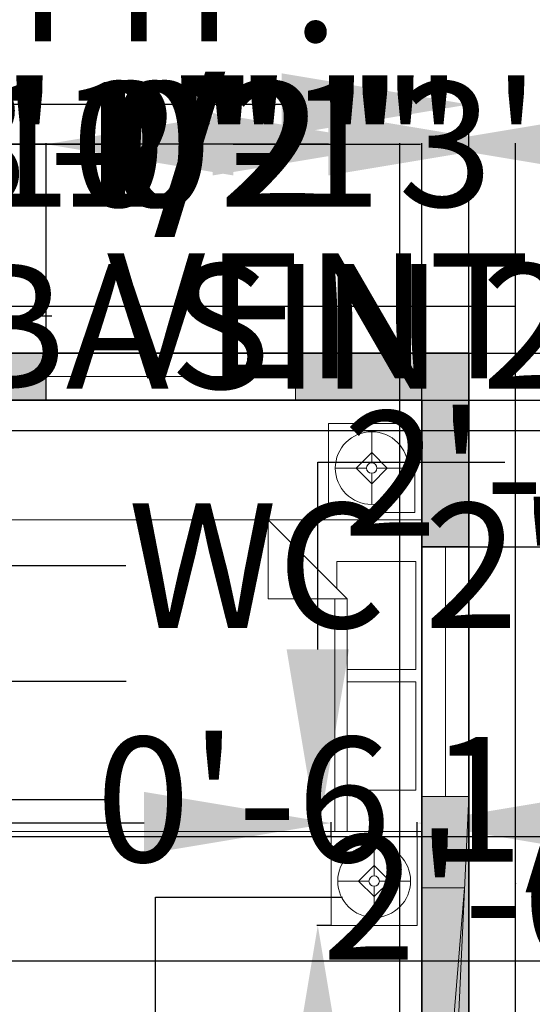
# Model space of a CAD drawing. Units: inches. Extents: x 2838 to 4029, y 1041 to 1915.
# Tile 13 of 16: x 3541 to 3640, y 1546 to 1735. Entities that reach past the tile are written whole.
import ezdxf

# ---------------------------------------------------------------- set-up
doc = ezdxf.new("R2010")
doc.units = ezdxf.units.IN
doc.header["$MEASUREMENT"] = 0
for name, color, linetype, lineweight in [('A-ANNO-DIMS', 2, 'Continuous', 18), ('A-FLOR', 7, 'Continuous', 25), ('A-FURN', 8, 'Continuous', 18), ('A-GLAZ', 4, 'Continuous', 18), ('A-REFR', 8, 'Continuous', 13), ('A-WALL', 7, 'Continuous', 35), ('A-WALL-PATT', 252, 'Continuous', 13)]:
    doc.layers.add(name, color=color, linetype=linetype, lineweight=lineweight)
doc.styles.get("Standard").update_dxf_attribs({"font": 'arial.ttf'})
doc.dimstyles.get("Standard").update_dxf_attribs({"dimtxt": 24, "dimasz": 36, "dimexe": 0.18, "dimexo": 0.0625, "dimgap": 0.09, "dimtad": 0, "dimtih": 1, "dimtoh": 1, "dimdec": 0, "dimzin": 0, "dimdsep": 46, "dimlunit": 3, "dimtxsty": 'Standard', "dimcen": 0.09, "dimadec": 0, "dimazin": 0, "dimtfac": 1, "dimtdec": 0, "dimtofl": 0, "dimtmove": 0, "dimatfit": 3, "dimfxl": 1, "dimtolj": 1, "dimtzin": 0, "dimarcsym": 0})

# ---------------------------------------------------------------- blocks, each defined once
blk = doc.blocks.new('Bed - Queen')
for p, q in [((0, -80.00003), (0, 0)), ((0, 0), (59.99999, 0)), ((59.99999, 0), (59.99999, -80.00003)), ((7.99999, -1.2), (28.79998, -1.2)), ((7.99999, -14.4), (7.99999, -1.2)), ((28.79998, -1.2), (28.79998, -14.4)), ((31.19999, -1.2), (51.99999, -1.2)), ((31.19999, -14.4), (31.19999, -1.2)), ((51.99999, -1.2), (51.99999, -16.4)), ((0, -14.4), (44.8, -14.4)), ((59.99999, -29.6), (44.8, -14.4)), ((44.8, -14.4), (44.8, -29.6)), ((44.8, -16.8), (0, -16.8)), ((51.99999, -16.4), (46.79936, -16.4)), ((44.8, -29.6), (59.99999, -29.6)), ((59.99999, -80.00003), (0, -80.00003))]:
    blk.add_line(p, q)
blk = doc.blocks.new('*D17')
at = {"layer": 'A-ANNO-DIMS', "color": 0, "lineweight": -2, "transparency": 16777216}
for p, q in [((3627.79, 1671.3), (3713.18, 1671.3)), ((3713, 1635.3), (3713, 1443.64)), ((3713, 1227.3), (3713, 1418.95)), ((3627.79, 1191.3), (3713.18, 1191.3))]:
    blk.add_line(p, q, dxfattribs=at)
at = {"layer": 'A-ANNO-DIMS', "color": 0, "transparency": 16777216}
for points in [[(3707, 1635.3), (3719, 1635.3), (3713, 1671.3)], [(3707, 1227.3), (3719, 1227.3), (3713, 1191.3)]]:
    blk.add_solid(points, dxfattribs=at)
at = {"layer": 'Defpoints', "color": 0, "transparency": 16777216}
for p in [(3627.73, 1671.3), (3627.73, 1191.3), (3713, 1191.3)]:
    blk.add_point(p, dxfattribs=at)
at = {"layer": 'A-ANNO-DIMS', "color": 0, "transparency": 16777216, "insert": (3713, 1431.3), "char_height": 24, "attachment_point": 5}
blk.add_mtext("\\A1;40'", dxfattribs=at)
blk = doc.blocks.new('*D18')
at = {"layer": 'A-ANNO-DIMS', "color": 0, "lineweight": -2, "transparency": 16777216}
for p, q in [((3267.73, 1671.36), (3267.73, 1719.35)), ((3303.73, 1719.17), (3427.28, 1719.17)), ((3591.73, 1719.17), (3468.18, 1719.17)), ((3627.73, 1671.36), (3627.73, 1719.35))]:
    blk.add_line(p, q, dxfattribs=at)
at = {"layer": 'A-ANNO-DIMS', "color": 0, "transparency": 16777216}
for points in [[(3303.73, 1725.17), (3303.73, 1713.17), (3267.73, 1719.17)], [(3591.73, 1725.17), (3591.73, 1713.17), (3627.73, 1719.17)]]:
    blk.add_solid(points, dxfattribs=at)
at = {"layer": 'Defpoints', "color": 0, "transparency": 16777216}
for p in [(3267.73, 1719.17), (3267.73, 1671.3), (3627.73, 1671.3)]:
    blk.add_point(p, dxfattribs=at)
at = {"layer": 'A-ANNO-DIMS', "color": 0, "transparency": 16777216, "insert": (3447.73, 1719.17), "char_height": 24, "attachment_point": 5}
blk.add_mtext("\\A1;30'", dxfattribs=at)
blk = doc.blocks.new('WIN-48')
blk.add_line((4.5, 48), (4.5, 0))
blk.add_lwpolyline([(0, 48), (9, 48), (9, 0), (0, 0)], close=True)
blk = doc.blocks.new('Lamp - Table')
for p, q in [((0, 7), (0, 1)), ((0, 3), (-3, 0)), ((3, 0), (0, 3)), ((-1, 0), (-7, 0)), ((-3, 0), (0, -3)), ((0, -3), (3, 0)), ((1, 0), (7, 0)), ((0, -1), (0, -7))]:
    blk.add_line(p, q)
for radius in [7, 1]:
    blk.add_circle((0, 0), radius)
blk = doc.blocks.new('NIGHTSTAND-WITH-LAMP')
blk.add_lwpolyline([(0, 17.15), (16.57, 17.15), (16.57, 0), (0, 0)], close=True)
blk.add_blockref('Lamp - Table', (8.28, 8.57))
blk = doc.blocks.new('*D27')
at = {"layer": 'A-ANNO-DIMS', "color": 0, "lineweight": -2, "transparency": 16777216}
for p, q in [((3598.68, 1614.31), (3598.68, 1650.31)), ((3598.68, 1650.31), (3634.68, 1650.31)), ((3601.19, 1578.31), (3598.5, 1578.31)), ((3601.19, 1561.16), (3598.5, 1561.16)), ((3598.68, 1525.16), (3598.68, 1489.16))]:
    blk.add_line(p, q, dxfattribs=at)
at = {"layer": 'A-ANNO-DIMS', "color": 0, "transparency": 16777216}
for points in [[(3592.68, 1614.31), (3604.68, 1614.31), (3598.68, 1578.31)], [(3592.68, 1525.16), (3604.68, 1525.16), (3598.68, 1561.16)]]:
    blk.add_solid(points, dxfattribs=at)
at = {"layer": 'Defpoints', "color": 0, "transparency": 16777216}
for p in [(3598.68, 1578.31), (3601.25, 1578.31), (3601.25, 1561.16)]:
    blk.add_point(p, dxfattribs=at)
at = {"layer": 'A-ANNO-DIMS', "color": 0, "transparency": 16777216, "insert": (3820.96, 1650.31), "char_height": 24, "attachment_point": 5}
blk.add_mtext('\\A1;NIGHTSTAND 1\'-5" TYP.', dxfattribs=at)
blk = doc.blocks.new('*D28')
at = {"layer": 'A-ANNO-DIMS', "color": 0, "lineweight": -2, "transparency": 16777216}
for p, q in [((3565.25, 1580.88), (3529.25, 1580.88)), ((3601.25, 1578.37), (3601.25, 1581.06)), ((3617.82, 1578.37), (3617.82, 1581.06)), ((3653.82, 1580.88), (3689.82, 1580.88))]:
    blk.add_line(p, q, dxfattribs=at)
at = {"layer": 'A-ANNO-DIMS', "color": 0, "transparency": 16777216}
for points in [[(3565.25, 1586.88), (3565.25, 1574.88), (3601.25, 1580.88)], [(3653.82, 1586.88), (3653.82, 1574.88), (3617.82, 1580.88)]]:
    blk.add_solid(points, dxfattribs=at)
at = {"layer": 'Defpoints', "color": 0, "transparency": 16777216}
for p in [(3617.82, 1580.88), (3601.25, 1578.31), (3617.82, 1578.31)]:
    blk.add_point(p, dxfattribs=at)
at = {"layer": 'A-ANNO-DIMS', "color": 0, "transparency": 16777216, "insert": (3789.89, 1580.88), "char_height": 24, "attachment_point": 5}
blk.add_mtext('\\A1;1\'-4 1/2" TYP.', dxfattribs=at)
blk = doc.blocks.new('*D36')
at = {"layer": 'A-ANNO-DIMS', "color": 0, "lineweight": -2, "transparency": 16777216}
for p, q in [((3481.95, 1586.87), (3481.95, 1585.25)), ((3488.45, 1586.87), (3488.45, 1585.25)), ((3445.95, 1585.43), (3409.95, 1585.43)), ((3524.45, 1585.43), (3560.45, 1585.43))]:
    blk.add_line(p, q, dxfattribs=at)
at = {"layer": 'A-ANNO-DIMS', "color": 0, "transparency": 16777216}
for points in [[(3445.95, 1591.43), (3445.95, 1579.43), (3481.95, 1585.43)], [(3524.45, 1591.43), (3524.45, 1579.43), (3488.45, 1585.43)]]:
    blk.add_solid(points, dxfattribs=at)
at = {"layer": 'Defpoints', "color": 0, "transparency": 16777216}
for p in [(3481.95, 1586.93), (3488.45, 1586.93), (3488.45, 1585.43)]:
    blk.add_point(p, dxfattribs=at)
at = {"layer": 'A-ANNO-DIMS', "color": 0, "transparency": 16777216, "insert": (3620.4, 1585.43), "char_height": 24, "attachment_point": 5}
blk.add_mtext('\\A1;0\'-6 1/2"', dxfattribs=at)
blk = doc.blocks.new('*D39')
at = {"layer": 'A-ANNO-DIMS', "color": 0, "lineweight": -2, "transparency": 16777216}
for p, q in [((3391.52, 1678.5), (3355.52, 1678.5)), ((3427.52, 1671.36), (3427.52, 1678.68)), ((3475.52, 1671.36), (3475.52, 1678.68)), ((3511.52, 1678.5), (3547.52, 1678.5))]:
    blk.add_line(p, q, dxfattribs=at)
at = {"layer": 'A-ANNO-DIMS', "color": 0, "transparency": 16777216}
for points in [[(3391.52, 1684.5), (3391.52, 1672.5), (3427.52, 1678.5)], [(3511.52, 1684.5), (3511.52, 1672.5), (3475.52, 1678.5)]]:
    blk.add_solid(points, dxfattribs=at)
at = {"layer": 'Defpoints', "color": 0, "transparency": 16777216}
for p in [(3475.52, 1678.5), (3427.52, 1671.3), (3475.52, 1671.3)]:
    blk.add_point(p, dxfattribs=at)
at = {"layer": 'A-ANNO-DIMS', "color": 0, "transparency": 16777216, "insert": (3732.24, 1678.5), "char_height": 24, "attachment_point": 5}
blk.add_mtext('\\A1;VENT BLOCK 4\'-0" TYP.', dxfattribs=at)
blk = doc.blocks.new('*D40')
at = {"layer": 'A-ANNO-DIMS', "color": 0, "lineweight": -2, "transparency": 16777216}
for p, q in [((3420.32, 1707.3), (3420.32, 1743.3)), ((3420.32, 1743.3), (3456.32, 1743.3)), ((3427.46, 1671.3), (3420.14, 1671.3)), ((3427.46, 1662.3), (3420.14, 1662.3)), ((3420.32, 1626.3), (3420.32, 1590.3))]:
    blk.add_line(p, q, dxfattribs=at)
at = {"layer": 'A-ANNO-DIMS', "color": 0, "transparency": 16777216}
for points in [[(3414.32, 1707.3), (3426.32, 1707.3), (3420.32, 1671.3)], [(3414.32, 1626.3), (3426.32, 1626.3), (3420.32, 1662.3)]]:
    blk.add_solid(points, dxfattribs=at)
at = {"layer": 'Defpoints', "color": 0, "transparency": 16777216}
for p in [(3420.32, 1671.3), (3427.52, 1671.3), (3427.52, 1662.3)]:
    blk.add_point(p, dxfattribs=at)
at = {"layer": 'A-ANNO-DIMS', "color": 0, "transparency": 16777216, "insert": (3529.56, 1743.3), "char_height": 24, "attachment_point": 5}
blk.add_mtext('\\A1;0\'-9" TYP.', dxfattribs=at)
blk = doc.blocks.new('*D41')
at = {"layer": 'A-ANNO-DIMS', "color": 0, "lineweight": -2, "transparency": 16777216}
for p, q in [((3284.24, 1506.2), (3284.24, 1496.56)), ((3347.73, 1506.2), (3347.73, 1496.56)), ((3248.24, 1496.74), (3212.24, 1496.74)), ((3383.73, 1496.74), (3419.73, 1496.74))]:
    blk.add_line(p, q, dxfattribs=at)
at = {"layer": 'A-ANNO-DIMS', "color": 0, "transparency": 16777216}
for points in [[(3248.24, 1502.74), (3248.24, 1490.74), (3284.24, 1496.74)], [(3383.73, 1502.74), (3383.73, 1490.74), (3347.73, 1496.74)]]:
    blk.add_solid(points, dxfattribs=at)
at = {"layer": 'Defpoints', "color": 0, "transparency": 16777216}
for p in [(3284.24, 1506.26), (3347.73, 1506.26), (3347.73, 1496.74)]:
    blk.add_point(p, dxfattribs=at)
at = {"layer": 'A-ANNO-DIMS', "color": 0, "transparency": 16777216, "insert": (3624.81, 1496.74), "char_height": 24, "attachment_point": 5}
blk.add_mtext('\\A1;WARDROBE 5\'-3 1/2" TYP.', dxfattribs=at)
blk = doc.blocks.new('*D45')
at = {"layer": 'A-ANNO-DIMS', "color": 0, "lineweight": -2, "transparency": 16777216}
for p, q in [((3456.69, 1635.35), (3456.69, 1630.27)), ((3489.73, 1635.35), (3489.73, 1630.27)), ((3420.69, 1630.45), (3384.69, 1630.45)), ((3525.73, 1630.45), (3561.73, 1630.45))]:
    blk.add_line(p, q, dxfattribs=at)
at = {"layer": 'A-ANNO-DIMS', "color": 0, "transparency": 16777216}
for points in [[(3420.69, 1636.45), (3420.69, 1624.45), (3456.69, 1630.45)], [(3525.73, 1636.45), (3525.73, 1624.45), (3489.73, 1630.45)]]:
    blk.add_solid(points, dxfattribs=at)
at = {"layer": 'Defpoints', "color": 0, "transparency": 16777216}
for p in [(3456.69, 1635.41), (3489.73, 1635.41), (3489.73, 1630.45)]:
    blk.add_point(p, dxfattribs=at)
at = {"layer": 'A-ANNO-DIMS', "color": 0, "transparency": 16777216, "insert": (3626.8, 1630.45), "char_height": 24, "attachment_point": 5}
blk.add_mtext('\\A1;WC 2\'-9"', dxfattribs=at)
blk = doc.blocks.new('*D47')
at = {"layer": 'A-ANNO-DIMS', "color": 0, "lineweight": -2, "transparency": 16777216}
for p, q in [((3493.47, 1640.5), (3493.47, 1676.5)), ((3493.47, 1676.5), (3529.47, 1676.5)), ((3489.85, 1604.5), (3493.65, 1604.5)), ((3489.85, 1579.95), (3493.65, 1579.95)), ((3493.47, 1543.95), (3493.47, 1507.95))]:
    blk.add_line(p, q, dxfattribs=at)
at = {"layer": 'A-ANNO-DIMS', "color": 0, "transparency": 16777216}
for points in [[(3487.47, 1640.5), (3499.47, 1640.5), (3493.47, 1604.5)], [(3487.47, 1543.95), (3499.47, 1543.95), (3493.47, 1579.95)]]:
    blk.add_solid(points, dxfattribs=at)
at = {"layer": 'Defpoints', "color": 0, "transparency": 16777216}
for p in [(3489.78, 1604.5), (3493.47, 1604.5), (3489.78, 1579.95)]:
    blk.add_point(p, dxfattribs=at)
at = {"layer": 'A-ANNO-DIMS', "color": 0, "transparency": 16777216, "insert": (3643.85, 1676.5), "char_height": 24, "attachment_point": 5}
blk.add_mtext('\\A1;BASIN 2\'-0 1/2"', dxfattribs=at)
blk = doc.blocks.new('*D48')
at = {"layer": 'A-ANNO-DIMS', "color": 0, "lineweight": -2, "transparency": 16777216}
for p, q in [((3433.65, 1608.18), (3397.65, 1608.18)), ((3469.65, 1604.56), (3469.65, 1608.36)), ((3489.78, 1604.56), (3489.78, 1608.36)), ((3525.78, 1608.18), (3561.78, 1608.18))]:
    blk.add_line(p, q, dxfattribs=at)
at = {"layer": 'A-ANNO-DIMS', "color": 0, "transparency": 16777216}
for points in [[(3433.65, 1614.18), (3433.65, 1602.18), (3469.65, 1608.18)], [(3525.78, 1614.18), (3525.78, 1602.18), (3489.78, 1608.18)]]:
    blk.add_solid(points, dxfattribs=at)
at = {"layer": 'Defpoints', "color": 0, "transparency": 16777216}
for p in [(3469.65, 1608.18), (3469.65, 1604.5), (3489.78, 1604.5)]:
    blk.add_point(p, dxfattribs=at)
at = {"layer": 'A-ANNO-DIMS', "color": 0, "transparency": 16777216, "insert": (3366.79, 1608.18), "char_height": 24, "attachment_point": 5}
blk.add_mtext('\\A1;1\'-8"', dxfattribs=at)
blk = doc.blocks.new('*D55')
at = {"layer": 'A-ANNO-DIMS', "color": 0, "lineweight": -2, "transparency": 16777216}
for p, q in [((3491.76, 1499.78), (3455.76, 1499.78)), ((3527.76, 1494.67), (3527.76, 1499.96)), ((3562.26, 1494.67), (3562.26, 1499.96)), ((3598.26, 1499.78), (3634.26, 1499.78))]:
    blk.add_line(p, q, dxfattribs=at)
at = {"layer": 'A-ANNO-DIMS', "color": 0, "transparency": 16777216}
for points in [[(3491.76, 1505.78), (3491.76, 1493.78), (3527.76, 1499.78)], [(3598.26, 1505.78), (3598.26, 1493.78), (3562.26, 1499.78)]]:
    blk.add_solid(points, dxfattribs=at)
at = {"layer": 'Defpoints', "color": 0, "transparency": 16777216}
for p in [(3527.76, 1499.78), (3527.76, 1494.6), (3562.26, 1494.6)]:
    blk.add_point(p, dxfattribs=at)
at = {"layer": 'A-ANNO-DIMS', "color": 0, "transparency": 16777216, "insert": (3260.33, 1499.78), "char_height": 24, "attachment_point": 5}
blk.add_mtext('\\A1;BASE CABINET 2\'-10 1/2"', dxfattribs=at)
blk = doc.blocks.new('*D56')
at = {"layer": 'A-ANNO-DIMS', "color": 0, "lineweight": -2, "transparency": 16777216}
for p, q in [((3567.44, 1530.6), (3567.44, 1566.6)), ((3567.44, 1566.6), (3603.44, 1566.6)), ((3562.33, 1494.6), (3567.62, 1494.6)), ((3562.33, 1470.6), (3567.62, 1470.6)), ((3567.44, 1434.6), (3567.44, 1398.6))]:
    blk.add_line(p, q, dxfattribs=at)
at = {"layer": 'A-ANNO-DIMS', "color": 0, "transparency": 16777216}
for points in [[(3561.44, 1530.6), (3573.44, 1530.6), (3567.44, 1494.6)], [(3561.44, 1434.6), (3573.44, 1434.6), (3567.44, 1470.6)]]:
    blk.add_solid(points, dxfattribs=at)
at = {"layer": 'Defpoints', "color": 0, "transparency": 16777216}
for p in [(3562.26, 1494.6), (3567.44, 1494.6), (3562.26, 1470.6)]:
    blk.add_point(p, dxfattribs=at)
at = {"layer": 'A-ANNO-DIMS', "color": 0, "transparency": 16777216, "insert": (3635.63, 1566.6), "char_height": 24, "attachment_point": 5}
blk.add_mtext('\\A1;2\'-0"', dxfattribs=at)
blk = doc.blocks.new('*D68')
at = {"layer": 'A-ANNO-DIMS', "color": 0, "lineweight": -2, "transparency": 16777216}
for p, q in [((3258.73, 1680.36), (3258.73, 1711.7)), ((3294.73, 1711.52), (3406.43, 1711.52)), ((3600.73, 1711.52), (3489.04, 1711.52)), ((3636.73, 1680.36), (3636.73, 1711.7))]:
    blk.add_line(p, q, dxfattribs=at)
at = {"layer": 'A-ANNO-DIMS', "color": 0, "transparency": 16777216}
for points in [[(3294.73, 1717.52), (3294.73, 1705.52), (3258.73, 1711.52)], [(3600.73, 1717.52), (3600.73, 1705.52), (3636.73, 1711.52)]]:
    blk.add_solid(points, dxfattribs=at)
at = {"layer": 'Defpoints', "color": 0, "transparency": 16777216}
for p in [(3636.73, 1711.52), (3258.73, 1680.3), (3636.73, 1680.3)]:
    blk.add_point(p, dxfattribs=at)
at = {"layer": 'A-ANNO-DIMS', "color": 0, "transparency": 16777216, "insert": (3447.73, 1711.52), "char_height": 24, "attachment_point": 5}
blk.add_mtext('\\A1;31\'-6"', dxfattribs=at)
blk = doc.blocks.new('*D73')
at = {"layer": 'A-ANNO-DIMS', "color": 0, "lineweight": -2, "transparency": 16777216}
for p, q in [((3425.038746, 1711.522346), (3389.038746, 1711.522346)), ((3461.038746, 1200.359846), (3461.038746, 1711.702346)), ((3618.731626, 1200.359846), (3618.731626, 1711.702346)), ((3654.731626, 1711.522346), (3690.731626, 1711.522346))]:
    blk.add_line(p, q, dxfattribs=at)
at = {"layer": 'A-ANNO-DIMS', "color": 0, "transparency": 16777216}
for points in [[(3425.038746, 1717.522346), (3425.038746, 1705.522346), (3461.038746, 1711.522346)], [(3654.731626, 1717.522346), (3654.731626, 1705.522346), (3618.731626, 1711.522346)]]:
    blk.add_solid(points, dxfattribs=at)
at = {"layer": 'Defpoints', "color": 0, "transparency": 16777216}
for p in [(3618.731626, 1711.522346), (3461.038746, 1200.297346), (3618.731626, 1200.297346)]:
    blk.add_point(p, dxfattribs=at)
at = {"layer": 'A-ANNO-DIMS', "color": 0, "transparency": 16777216, "insert": (3539.885186, 1711.522346), "char_height": 24, "attachment_point": 5}
blk.add_mtext('\\A1;13\'-1 1/2"', dxfattribs=at)
blk = doc.blocks.new('*D78')
at = {"layer": 'A-ANNO-DIMS', "color": 0, "lineweight": -2, "transparency": 16777216}
for p, q in [((3667.956626, 1590.394218), (3667.956626, 1626.394218)), ((3498.794126, 1554.394218), (3668.136626, 1554.394218)), ((3498.638013, 1506.394218), (3668.136626, 1506.394218)), ((3667.956626, 1470.394218), (3667.956626, 1434.394218))]:
    blk.add_line(p, q, dxfattribs=at)
at = {"layer": 'A-ANNO-DIMS', "color": 0, "transparency": 16777216}
for points in [[(3661.956626, 1590.394218), (3673.956626, 1590.394218), (3667.956626, 1554.394218)], [(3661.956626, 1470.394218), (3673.956626, 1470.394218), (3667.956626, 1506.394218)]]:
    blk.add_solid(points, dxfattribs=at)
at = {"layer": 'Defpoints', "color": 0, "transparency": 16777216}
for p in [(3498.731626, 1554.394218), (3667.956626, 1554.394218), (3498.575513, 1506.394218)]:
    blk.add_point(p, dxfattribs=at)
at = {"layer": 'A-ANNO-DIMS', "color": 0, "transparency": 16777216, "insert": (3667.956626, 1530.394218), "char_height": 24, "attachment_point": 5}
blk.add_mtext('\\A1;4\'-0"', dxfattribs=at)
blk = doc.blocks.new('*D79')
at = {"layer": 'A-ANNO-DIMS', "color": 0, "lineweight": -2, "transparency": 16777216}
for p, q in [((3379.05, 1400.64), (3379.05, 1711.7)), ((3415.05, 1711.52), (3418.63, 1711.52)), ((3454.63, 1398.31), (3454.63, 1711.7)), ((3454.63, 1711.52), (3490.63, 1711.52))]:
    blk.add_line(p, q, dxfattribs=at)
at = {"layer": 'A-ANNO-DIMS', "color": 0, "transparency": 16777216}
for points in [[(3415.05, 1717.52), (3415.05, 1705.52), (3379.05, 1711.52)], [(3418.63, 1717.52), (3418.63, 1705.52), (3454.63, 1711.52)]]:
    blk.add_solid(points, dxfattribs=at)
at = {"layer": 'Defpoints', "color": 0, "transparency": 16777216}
for p in [(3454.63, 1711.52), (3379.05, 1400.57), (3454.63, 1398.25)]:
    blk.add_point(p, dxfattribs=at)
at = {"layer": 'A-ANNO-DIMS', "color": 0, "transparency": 16777216, "insert": (3550.65, 1711.52), "char_height": 24, "attachment_point": 5}
blk.add_mtext('\\A1;6\'-3 1/2"', dxfattribs=at)
blk = doc.blocks.new('*D82')
at = {"layer": 'A-ANNO-DIMS', "color": 0, "lineweight": -2, "transparency": 16777216}
for p, q in [((3405.73, 1573.06), (3405.73, 1081.89)), ((3441.73, 1569.23), (3441.73, 1081.89)), ((3369.73, 1082.07), (3333.73, 1082.07)), ((3477.73, 1082.07), (3513.73, 1082.07))]:
    blk.add_line(p, q, dxfattribs=at)
at = {"layer": 'A-ANNO-DIMS', "color": 0, "transparency": 16777216}
for points in [[(3369.73, 1088.07), (3369.73, 1076.07), (3405.73, 1082.07)], [(3477.73, 1088.07), (3477.73, 1076.07), (3441.73, 1082.07)]]:
    blk.add_solid(points, dxfattribs=at)
at = {"layer": 'Defpoints', "color": 0, "transparency": 16777216}
for p in [(3405.73, 1573.12), (3441.73, 1569.3), (3441.73, 1082.07)]:
    blk.add_point(p, dxfattribs=at)
at = {"layer": 'A-ANNO-DIMS', "color": 0, "transparency": 16777216, "insert": (3545.71, 1082.07), "char_height": 24, "attachment_point": 5}
blk.add_mtext('\\A1;3\'-0"', dxfattribs=at)
blk = doc.blocks.new('*D83')
at = {"layer": 'A-ANNO-DIMS', "color": 0, "lineweight": -2, "transparency": 16777216}
for p, q in [((3405.73, 1662.36), (3405.73, 1711.7)), ((3441.73, 1711.52), (3453.73, 1711.52)), ((3489.73, 1662.36), (3489.73, 1711.7)), ((3489.73, 1711.52), (3525.73, 1711.52))]:
    blk.add_line(p, q, dxfattribs=at)
at = {"layer": 'A-ANNO-DIMS', "color": 0, "transparency": 16777216}
for points in [[(3441.73, 1717.52), (3441.73, 1705.52), (3405.73, 1711.52)], [(3453.73, 1717.52), (3453.73, 1705.52), (3489.73, 1711.52)]]:
    blk.add_solid(points, dxfattribs=at)
at = {"layer": 'Defpoints', "color": 0, "transparency": 16777216}
for p in [(3489.73, 1711.52), (3405.73, 1662.3), (3489.73, 1662.3)]:
    blk.add_point(p, dxfattribs=at)
at = {"layer": 'A-ANNO-DIMS', "color": 0, "transparency": 16777216, "insert": (3557.62, 1711.52), "char_height": 24, "attachment_point": 5}
blk.add_mtext('\\A1;7\'-0"', dxfattribs=at)
blk = doc.blocks.new('*D84')
at = {"layer": 'A-ANNO-DIMS', "color": 0, "lineweight": -2, "transparency": 16777216}
for p, q in [((3667.96, 1662.3), (3667.96, 1698.3)), ((3667.96, 1698.3), (3703.96, 1698.3)), ((3489.79, 1662.3), (3668.14, 1662.3)), ((3667.96, 1614.3), (3667.96, 1626.3)), ((3489.79, 1578.3), (3668.14, 1578.3))]:
    blk.add_line(p, q, dxfattribs=at)
at = {"layer": 'A-ANNO-DIMS', "color": 0, "transparency": 16777216}
for points in [[(3661.96, 1626.3), (3673.96, 1626.3), (3667.96, 1662.3)], [(3661.96, 1614.3), (3673.96, 1614.3), (3667.96, 1578.3)]]:
    blk.add_solid(points, dxfattribs=at)
at = {"layer": 'Defpoints', "color": 0, "transparency": 16777216}
for p in [(3489.73, 1662.3), (3667.96, 1662.3), (3489.73, 1578.3)]:
    blk.add_point(p, dxfattribs=at)
at = {"layer": 'A-ANNO-DIMS', "color": 0, "transparency": 16777216, "insert": (3735.85, 1698.3), "char_height": 24, "attachment_point": 5}
blk.add_mtext('\\A1;7\'-0"', dxfattribs=at)
blk = doc.blocks.new('*D85')
at = {"layer": 'A-ANNO-DIMS', "color": 0, "lineweight": -2, "transparency": 16777216}
for p, q in [((3369.73, 1711.52), (3333.73, 1711.52)), ((3405.73, 1662.36), (3405.73, 1711.7)), ((3427.52, 1662.36), (3427.52, 1711.7)), ((3463.52, 1711.52), (3499.52, 1711.52))]:
    blk.add_line(p, q, dxfattribs=at)
at = {"layer": 'A-ANNO-DIMS', "color": 0, "transparency": 16777216}
for points in [[(3369.73, 1717.52), (3369.73, 1705.52), (3405.73, 1711.52)], [(3463.52, 1717.52), (3463.52, 1705.52), (3427.52, 1711.52)]]:
    blk.add_solid(points, dxfattribs=at)
at = {"layer": 'Defpoints', "color": 0, "transparency": 16777216}
for p in [(3427.52, 1711.52), (3405.73, 1662.3), (3427.52, 1662.3)]:
    blk.add_point(p, dxfattribs=at)
at = {"layer": 'A-ANNO-DIMS', "color": 0, "transparency": 16777216, "insert": (3539.7, 1711.52), "char_height": 24, "attachment_point": 5}
blk.add_mtext('\\A1;1\'-10"', dxfattribs=at)
blk = doc.blocks.new('*D86')
at = {"layer": 'A-ANNO-DIMS', "color": 0, "lineweight": -2, "transparency": 16777216}
for p, q in [((3391.52, 1711.52), (3355.52, 1711.52)), ((3427.52, 1671.36), (3427.52, 1711.7)), ((3451.52, 1671.36), (3451.52, 1711.7)), ((3487.52, 1711.52), (3523.52, 1711.52))]:
    blk.add_line(p, q, dxfattribs=at)
at = {"layer": 'A-ANNO-DIMS', "color": 0, "transparency": 16777216}
for points in [[(3391.52, 1717.52), (3391.52, 1705.52), (3427.52, 1711.52)], [(3487.52, 1717.52), (3487.52, 1705.52), (3451.52, 1711.52)]]:
    blk.add_solid(points, dxfattribs=at)
at = {"layer": 'Defpoints', "color": 0, "transparency": 16777216}
for p in [(3451.52, 1711.52), (3427.52, 1671.3), (3451.52, 1671.3)]:
    blk.add_point(p, dxfattribs=at)
at = {"layer": 'A-ANNO-DIMS', "color": 0, "transparency": 16777216, "insert": (3555.72, 1711.52), "char_height": 24, "attachment_point": 5}
blk.add_mtext('\\A1;2\'-0"', dxfattribs=at)
blk = doc.blocks.new('*D94')
at = {"layer": 'A-ANNO-DIMS', "color": 0, "lineweight": -2, "transparency": 16777216}
for p, q in [((3667.96, 1533.39), (3667.96, 1569.39)), ((3585.44, 1497.39), (3668.14, 1497.39)), ((3585.44, 1469.25), (3668.14, 1469.25)), ((3667.96, 1433.25), (3667.96, 1397.25))]:
    blk.add_line(p, q, dxfattribs=at)
at = {"layer": 'A-ANNO-DIMS', "color": 0, "transparency": 16777216}
for points in [[(3661.96, 1533.39), (3673.96, 1533.39), (3667.96, 1497.39)], [(3661.96, 1433.25), (3673.96, 1433.25), (3667.96, 1469.25)]]:
    blk.add_solid(points, dxfattribs=at)
at = {"layer": 'Defpoints', "color": 0, "transparency": 16777216}
for p in [(3585.37, 1497.39), (3585.37, 1469.25), (3667.96, 1469.25)]:
    blk.add_point(p, dxfattribs=at)
at = {"layer": 'A-ANNO-DIMS', "color": 0, "transparency": 16777216, "insert": (3667.96, 1483.32), "char_height": 24, "attachment_point": 5}
blk.add_mtext('\\A1;2\'-4"', dxfattribs=at)
blk = doc.blocks.new('*D96')
at = {"layer": 'A-ANNO-DIMS', "color": 0, "lineweight": -2, "transparency": 16777216}
for p, q in [((3462.73, 1711.52), (3426.73, 1711.52)), ((3498.73, 1662.36), (3498.73, 1711.7)), ((3546.42, 1662.36), (3546.42, 1711.7)), ((3582.42, 1711.52), (3618.42, 1711.52))]:
    blk.add_line(p, q, dxfattribs=at)
at = {"layer": 'A-ANNO-DIMS', "color": 0, "transparency": 16777216}
for points in [[(3462.73, 1717.52), (3462.73, 1705.52), (3498.73, 1711.52)], [(3582.42, 1717.52), (3582.42, 1705.52), (3546.42, 1711.52)]]:
    blk.add_solid(points, dxfattribs=at)
at = {"layer": 'Defpoints', "color": 0, "transparency": 16777216}
for p in [(3546.42, 1711.52), (3498.73, 1662.3), (3546.42, 1662.3)]:
    blk.add_point(p, dxfattribs=at)
at = {"layer": 'A-ANNO-DIMS', "color": 0, "transparency": 16777216, "insert": (3687.68, 1711.52), "char_height": 24, "attachment_point": 5}
blk.add_mtext('\\A1;3\'-11 1/2"', dxfattribs=at)
blk = doc.blocks.new('*D97')
at = {"layer": 'A-ANNO-DIMS', "color": 0, "lineweight": -2, "transparency": 16777216}
for p, q in [((3667.956626, 1698.297346), (3667.956626, 1734.297346)), ((3618.794126, 1662.297346), (3668.136626, 1662.297346)), ((3618.794126, 1634.032994), (3668.136626, 1634.032994)), ((3667.956626, 1598.032994), (3667.956626, 1562.032994))]:
    blk.add_line(p, q, dxfattribs=at)
at = {"layer": 'A-ANNO-DIMS', "color": 0, "transparency": 16777216}
for points in [[(3661.956626, 1698.297346), (3673.956626, 1698.297346), (3667.956626, 1662.297346)], [(3661.956626, 1598.032994), (3673.956626, 1598.032994), (3667.956626, 1634.032994)]]:
    blk.add_solid(points, dxfattribs=at)
at = {"layer": 'Defpoints', "color": 0, "transparency": 16777216}
for p in [(3618.731626, 1662.297346), (3618.731626, 1634.032994), (3667.956626, 1634.032994)]:
    blk.add_point(p, dxfattribs=at)
at = {"layer": 'A-ANNO-DIMS', "color": 0, "transparency": 16777216, "insert": (3667.956626, 1648.16517), "char_height": 24, "attachment_point": 5}
blk.add_mtext('\\A1;2\'-4 1/2"', dxfattribs=at)
blk = doc.blocks.new('*D101')
at = {"layer": 'A-ANNO-DIMS', "color": 0, "lineweight": -2, "transparency": 16777216}
for p, q in [((3425.04, 1711.52), (3389.04, 1711.52)), ((3461.04, 1200.36), (3461.04, 1711.7)), ((3486.18, 1200.36), (3486.18, 1711.7)), ((3522.18, 1711.52), (3558.18, 1711.52))]:
    blk.add_line(p, q, dxfattribs=at)
at = {"layer": 'A-ANNO-DIMS', "color": 0, "transparency": 16777216}
for points in [[(3425.04, 1717.52), (3425.04, 1705.52), (3461.04, 1711.52)], [(3522.18, 1717.52), (3522.18, 1705.52), (3486.18, 1711.52)]]:
    blk.add_solid(points, dxfattribs=at)
at = {"layer": 'Defpoints', "color": 0, "transparency": 16777216}
for p in [(3486.18, 1711.52), (3461.04, 1200.3), (3486.18, 1200.3)]:
    blk.add_point(p, dxfattribs=at)
at = {"layer": 'A-ANNO-DIMS', "color": 0, "transparency": 16777216, "insert": (3590.37, 1711.52), "char_height": 24, "attachment_point": 5}
blk.add_mtext('\\A1;2\'-1"', dxfattribs=at)
blk = doc.blocks.new('*D102')
at = {"layer": 'A-ANNO-DIMS', "color": 0, "lineweight": -2, "transparency": 16777216}
for p, q in [((3667.96, 1698.3), (3667.96, 1734.3)), ((3667.96, 1734.3), (3703.96, 1734.3)), ((3489.79, 1662.3), (3668.14, 1662.3)), ((3489.79, 1656.41), (3668.14, 1656.41)), ((3667.96, 1620.41), (3667.96, 1584.41))]:
    blk.add_line(p, q, dxfattribs=at)
at = {"layer": 'A-ANNO-DIMS', "color": 0, "transparency": 16777216}
for points in [[(3661.96, 1698.3), (3673.96, 1698.3), (3667.96, 1662.3)], [(3661.96, 1620.41), (3673.96, 1620.41), (3667.96, 1656.41)]]:
    blk.add_solid(points, dxfattribs=at)
at = {"layer": 'Defpoints', "color": 0, "transparency": 16777216}
for p in [(3489.73, 1662.3), (3667.96, 1662.3), (3489.73, 1656.41)]:
    blk.add_point(p, dxfattribs=at)
at = {"layer": 'A-ANNO-DIMS', "color": 0, "transparency": 16777216, "insert": (3735.95, 1734.3), "char_height": 24, "attachment_point": 5}
blk.add_mtext('\\A1;0\'-6"', dxfattribs=at)
blk = doc.blocks.new('*D104')
at = {"layer": 'A-ANNO-DIMS', "color": 0, "lineweight": -2, "transparency": 16777216}
for p, q in [((3667.956626, 1533.394218), (3667.956626, 1569.394218)), ((3618.794126, 1497.394218), (3668.136626, 1497.394218)), ((3614.522024, 1472.357294), (3668.136626, 1472.357294)), ((3667.956626, 1436.357294), (3667.956626, 1400.357294))]:
    blk.add_line(p, q, dxfattribs=at)
at = {"layer": 'A-ANNO-DIMS', "color": 0, "transparency": 16777216}
for points in [[(3661.956626, 1533.394218), (3673.956626, 1533.394218), (3667.956626, 1497.394218)], [(3661.956626, 1436.357294), (3673.956626, 1436.357294), (3667.956626, 1472.357294)]]:
    blk.add_solid(points, dxfattribs=at)
at = {"layer": 'Defpoints', "color": 0, "transparency": 16777216}
for p in [(3618.731626, 1497.394218), (3614.459524, 1472.357294), (3667.956626, 1472.357294)]:
    blk.add_point(p, dxfattribs=at)
at = {"layer": 'A-ANNO-DIMS', "color": 0, "transparency": 16777216, "insert": (3667.956626, 1484.875756), "char_height": 24, "attachment_point": 5}
blk.add_mtext('\\A1;2\'-1"', dxfattribs=at)
blk = doc.blocks.new('*D105')
at = {"layer": 'A-ANNO-DIMS', "color": 0, "lineweight": -2, "transparency": 16777216}
for p, q in [((3578.46, 1711.52), (3542.46, 1711.52)), ((3614.46, 1472.42), (3614.46, 1711.7)), ((3618.73, 1469.91), (3618.73, 1711.7)), ((3654.73, 1711.52), (3690.73, 1711.52))]:
    blk.add_line(p, q, dxfattribs=at)
at = {"layer": 'A-ANNO-DIMS', "color": 0, "transparency": 16777216}
for points in [[(3578.46, 1717.52), (3578.46, 1705.52), (3614.46, 1711.52)], [(3654.73, 1717.52), (3654.73, 1705.52), (3618.73, 1711.52)]]:
    blk.add_solid(points, dxfattribs=at)
at = {"layer": 'Defpoints', "color": 0, "transparency": 16777216}
for p in [(3618.73, 1711.52), (3614.46, 1472.36), (3618.73, 1469.85)]:
    blk.add_point(p, dxfattribs=at)
at = {"layer": 'A-ANNO-DIMS', "color": 0, "transparency": 16777216, "insert": (3750.68, 1711.52), "char_height": 24, "attachment_point": 5}
blk.add_mtext('\\A1;0\'-4 1/2"', dxfattribs=at)

msp = doc.modelspace()

# ---------------------------------------------------------------- hatches: boundary and pattern name
at = {"layer": 'A-WALL-PATT'}
h = msp.add_hatch(color=256, dxfattribs=at)
h.dxf.hatch_style = 1
h.paths.add_polyline_path([(3427.52, 1671.3), (3360.91, 1671.3), (3360.91, 1662.3), (3396.73, 1662.3), (3396.73, 1554.39), (3397.12, 1554.39, -0.007312), (3398.53, 1554.41), (3405.73, 1554.41), (3405.73, 1662.3), (3427.52, 1662.3)])
h.paths.add_polyline_path([(3546.42, 1671.3), (3451.52, 1671.3), (3451.52, 1662.3), (3489.73, 1662.3), (3489.73, 1592.86, -0.016107), (3489.73, 1591.9), (3489.73, 1578.3), (3441.73, 1578.3), (3441.73, 1569.3), (3489.73, 1569.3), (3489.73, 1554.41), (3498.73, 1554.41), (3498.73, 1662.3), (3546.42, 1662.3)])
h.paths.add_polyline_path([(3627.73, 1671.3), (3594.42, 1671.3), (3594.42, 1662.3), (3618.73, 1662.3), (3618.73, 1634.03), (3627.73, 1634.03)])
h.paths.add_polyline_path([(3627.73, 1586.03), (3618.73, 1586.03), (3618.73, 1506.39), (3545.12, 1506.39), (3489.73, 1506.39), (3489.73, 1497.39), (3513.73, 1497.39), (3618.73, 1497.39), (3618.73, 1469.85), (3627.73, 1469.85)])
h.paths.add_polyline_path([(3627.73, 1421.85), (3618.73, 1421.85), (3618.73, 1378.73), (3522.73, 1378.73), (3513.73, 1378.73), (3461.04, 1378.73), (3461.04, 1369.73), (3513.73, 1369.73), (3618.73, 1369.73), (3618.73, 1320.94), (3627.73, 1320.94)])
h.paths.add_polyline_path([(3627.73, 1272.94), (3618.73, 1272.94), (3618.73, 1200.3), (3599.07, 1200.3), (3599.07, 1191.3), (3627.73, 1191.3)])
h.paths.add_polyline_path([(3551.07, 1200.3), (3510.18, 1200.3), (3510.18, 1191.3), (3551.07, 1191.3)])
h.paths.add_polyline_path([(3486.18, 1200.3), (3461.04, 1200.3), (3461.04, 1398.25), (3454.63, 1398.25), (3454.63, 1200.3), (3432.45, 1200.3), (3432.45, 1191.3), (3486.18, 1191.3)])
h.paths.add_polyline_path([(3300.73, 1200.3), (3276.73, 1200.3), (3276.73, 1391.57), (3331.05, 1391.57), (3331.05, 1400.57), (3276.73, 1400.57), (3276.73, 1432.17), (3267.73, 1432.17), (3267.73, 1191.3), (3300.73, 1191.3)])

# ---------------------------------------------------------------- linework, layer by layer
at = {"layer": 'A-FLOR'}
msp.add_lwpolyline([(3527.95, 1182.3), (3636.73, 1182.3), (3636.73, 1680.3), (3258.73, 1680.3), (3258.73, 1182.3), (3267.73, 1182.3)], dxfattribs=at)
at = {"layer": 'A-REFR'}
for p, q in [((3627.73, 1586.03), (3623.23, 1488.12)), ((3627.73, 1469.85), (3627.73, 1586.03)), ((3626.92, 1568.43), (3618.73, 1568.43)), ((3621.1, 1497.39), (3626.92, 1568.43))]:
    msp.add_line(p, q, dxfattribs=at)
msp.add_point((3636.73, 1569.29), dxfattribs=at)
at = {"layer": 'A-WALL'}
for p, q in [((3627.73, 1671.3), (3267.73, 1671.3)), ((3627.73, 1191.3), (3627.73, 1671.3)), ((3618.73, 1662.3), (3498.73, 1662.3)), ((3498.73, 1662.3), (3618.73, 1662.3)), ((3618.73, 1506.39), (3618.73, 1662.3)), ((3618.73, 1662.3), (3618.73, 1634.03)), ((3618.73, 1634.03), (3618.73, 1586.03)), ((3627.73, 1634.03), (3618.73, 1634.03)), ((3627.73, 1586.03), (3627.73, 1634.03)), ((3618.73, 1586.03), (3618.73, 1506.39)), ((3627.73, 1421.85), (3627.73, 1586.03))]:
    msp.add_line(p, q, dxfattribs=at)
msp.add_lwpolyline([(3372.73, 1191.3), (3627.73, 1191.3), (3627.73, 1671.3), (3267.73, 1671.3), (3267.73, 1191.3), (3300.73, 1191.3)], dxfattribs=at)

# ---------------------------------------------------------------- block references
at = {"layer": 'A-FURN'}
for p in [(3600.77, 1640.63), (3601.25, 1561.16)]:
    msp.add_blockref('NIGHTSTAND-WITH-LAMP', p, dxfattribs=at)
at = {"layer": 'A-FURN', "xscale": -1, "rotation": 270}
msp.add_blockref('Bed - Queen', (3618.73, 1579.24), dxfattribs=at)
at = {"layer": 'A-GLAZ', "rotation": 269.999999999997}
msp.add_blockref('WIN-48', (3546.42, 1671.3), dxfattribs=at)
at = {"layer": 'A-GLAZ'}
msp.add_blockref('WIN-48', (3618.73, 1586.03), dxfattribs=at)

# ---------------------------------------------------------------- dimensions: what is measured, and where the dimension line sits
at = {"layer": 'A-ANNO-DIMS'}
for base, p1, p2, angle, text, picture, middle in [((3420.32, 1671.3), (3427.52, 1662.3), (3427.52, 1671.3), 90, '<> TYP.', '*D40', (3529.56, 1743.3)), ((3493.4667, 1604.5013), (3489.7841, 1579.9504), (3489.7841, 1604.5013), 90, 'BASIN <>', '*D47', (3643.8514, 1676.5013)), ((3598.6826, 1578.3092), (3601.2549, 1561.1604), (3601.2549, 1578.3092), 90, 'NIGHTSTAND <> TYP.', '*D27', (3820.9609, 1650.3092)), ((3527.76, 1499.78), (3562.26, 1494.6), (3527.76, 1494.6), 180, 'BASE CABINET <>', '*D55', (3260.33, 1499.78))]:
    dim = msp.add_linear_dim(base=base, p1=p1, p2=p2, angle=angle, text=text, dimstyle='Standard', override={"dimdec": 1, "dimlfac": 1, "dimrnd": 0, "dimzin": 1, "dimdsep": 46, "dimlunit": 4, "dimfrac": 2}, dxfattribs=at)
    dim.commit()
    dim.dimension.update_dxf_attribs({"geometry": picture, "text_midpoint": middle})
for base, p1, p2, text, picture, middle in [((3475.52, 1678.5), (3427.52, 1671.3), (3475.52, 1671.3), 'VENT BLOCK <> TYP.', '*D39', (3732.24, 1678.5)), ((3489.73, 1630.45), (3456.69, 1635.41), (3489.73, 1635.41), 'WC <>', '*D45', (3626.8, 1630.45)), ((3617.82, 1580.88), (3601.25, 1578.31), (3617.82, 1578.31), '<> TYP.', '*D28', (3789.89, 1580.88)), ((3347.73, 1496.74), (3284.24, 1506.26), (3347.73, 1506.26), 'WARDROBE <> TYP.', '*D41', (3624.81, 1496.74))]:
    dim = msp.add_linear_dim(base=base, p1=p1, p2=p2, text=text, dimstyle='Standard', override={"dimdec": 1, "dimlfac": 1, "dimrnd": 0, "dimzin": 1, "dimdsep": 46, "dimlunit": 4, "dimfrac": 2}, dxfattribs=at)
    dim.commit()
    dim.dimension.update_dxf_attribs({"geometry": picture, "text_midpoint": middle})
for base, p1, p2, angle, override, picture, middle in [((3667.96, 1662.3), (3489.73, 1656.41), (3489.73, 1662.3), 90, {"dimdec": 1, "dimlfac": 1, "dimrnd": 0, "dimzin": 1, "dimdsep": 46, "dimlunit": 4, "dimfrac": 2}, '*D102', (3735.95, 1734.3)), ((3667.96, 1634.03), (3618.73, 1662.3), (3618.73, 1634.03), 90, {"dimdec": 1, "dimlfac": 1, "dimrnd": 0, "dimzin": 1, "dimdsep": 46, "dimlunit": 4, "dimfrac": 2}, '*D97', (3667.96, 1648.17)), ((3667.96, 1662.3), (3489.73, 1578.3), (3489.73, 1662.3), 90, {"dimdec": 1, "dimlfac": 1, "dimrnd": 0, "dimzin": 1, "dimdsep": 46, "dimlunit": 4, "dimfrac": 2}, '*D84', (3735.85, 1698.3)), ((3713, 1191.3), (3627.73, 1671.3), (3627.73, 1191.3), 90, {"dimclrd": 0, "dimclre": 0, "dimclrt": 0}, '*D17', (3713, 1431.3)), ((3667.96, 1554.39), (3498.58, 1506.39), (3498.73, 1554.39), 90, {"dimdec": 1, "dimlfac": 1, "dimrnd": 0, "dimzin": 1, "dimdsep": 46, "dimlunit": 4, "dimfrac": 2}, '*D78', (3667.96, 1530.39)), ((3469.65, 1608.18), (3489.78, 1604.5), (3469.65, 1604.5), 180, {"dimdec": 1, "dimlfac": 1, "dimrnd": 0, "dimzin": 1, "dimdsep": 46, "dimlunit": 4, "dimfrac": 2}, '*D48', (3366.79, 1608.18)), ((3567.44, 1494.6), (3562.26, 1470.6), (3562.26, 1494.6), 90, {"dimdec": 1, "dimlfac": 1, "dimrnd": 0, "dimzin": 1, "dimdsep": 46, "dimlunit": 4, "dimfrac": 2}, '*D56', (3635.63, 1566.6)), ((3667.96, 1469.25), (3585.37, 1497.39), (3585.37, 1469.25), 90, {"dimdec": 1, "dimlfac": 1, "dimrnd": 0, "dimzin": 1, "dimdsep": 46, "dimlunit": 4, "dimfrac": 2}, '*D94', (3667.96, 1483.32)), ((3667.96, 1472.36), (3618.73, 1497.39), (3614.46, 1472.36), 90, {"dimdec": 1, "dimlfac": 1, "dimrnd": 0, "dimzin": 1, "dimdsep": 46, "dimlunit": 4, "dimfrac": 2}, '*D104', (3667.96, 1484.88))]:
    dim = msp.add_linear_dim(base=base, p1=p1, p2=p2, angle=angle, dimstyle='Standard', override=override, dxfattribs=at)
    dim.commit()
    dim.dimension.update_dxf_attribs({"geometry": picture, "text_midpoint": middle})
for base, p1, p2, override, picture, middle in [((3454.63, 1711.52), (3379.05, 1400.57), (3454.63, 1398.25), {"dimdec": 1, "dimlfac": 1, "dimrnd": 0, "dimzin": 1, "dimdsep": 46, "dimlunit": 4, "dimfrac": 2}, '*D79', (3550.65, 1711.52)), ((3618.73, 1711.52), (3461.04, 1200.3), (3618.73, 1200.3), {"dimdec": 1, "dimlfac": 1, "dimrnd": 0, "dimzin": 1, "dimdsep": 46, "dimlunit": 4, "dimfrac": 2}, '*D73', (3539.89, 1711.52)), ((3546.42, 1711.52), (3498.73, 1662.3), (3546.42, 1662.3), {"dimdec": 1, "dimlfac": 1, "dimrnd": 0, "dimzin": 1, "dimdsep": 46, "dimlunit": 4, "dimfrac": 2}, '*D96', (3687.68, 1711.52)), ((3618.73, 1711.52), (3614.46, 1472.36), (3618.73, 1469.85), {"dimdec": 1, "dimlfac": 1, "dimrnd": 0, "dimzin": 1, "dimdsep": 46, "dimlunit": 4, "dimfrac": 2}, '*D105', (3750.68, 1711.52)), ((3267.73, 1719.17), (3627.73, 1671.3), (3267.73, 1671.3), {"dimclrd": 0, "dimclre": 0, "dimclrt": 0}, '*D18', (3447.73, 1719.17)), ((3636.73, 1711.52), (3258.73, 1680.3), (3636.73, 1680.3), {"dimdec": 1, "dimlfac": 1, "dimrnd": 0, "dimzin": 1, "dimdsep": 46, "dimlunit": 4, "dimfrac": 2}, '*D68', (3447.73, 1711.52)), ((3427.52, 1711.52), (3405.73, 1662.3), (3427.52, 1662.3), {"dimdec": 1, "dimlfac": 1, "dimrnd": 0, "dimzin": 1, "dimdsep": 46, "dimlunit": 4, "dimfrac": 2}, '*D85', (3539.7, 1711.52)), ((3451.52, 1711.52), (3427.52, 1671.3), (3451.52, 1671.3), {"dimdec": 1, "dimlfac": 1, "dimrnd": 0, "dimzin": 1, "dimdsep": 46, "dimlunit": 4, "dimfrac": 2}, '*D86', (3555.72, 1711.52)), ((3486.18, 1711.52), (3461.04, 1200.3), (3486.18, 1200.3), {"dimdec": 1, "dimlfac": 1, "dimrnd": 0, "dimzin": 1, "dimdsep": 46, "dimlunit": 4, "dimfrac": 2}, '*D101', (3590.37, 1711.52)), ((3489.73, 1711.52), (3405.73, 1662.3), (3489.73, 1662.3), {"dimdec": 1, "dimlfac": 1, "dimrnd": 0, "dimzin": 1, "dimdsep": 46, "dimlunit": 4, "dimfrac": 2}, '*D83', (3557.62, 1711.52)), ((3488.45, 1585.43), (3481.95, 1586.93), (3488.45, 1586.93), {"dimdec": 1, "dimlfac": 1, "dimrnd": 0, "dimzin": 1, "dimdsep": 46, "dimlunit": 4, "dimfrac": 2}, '*D36', (3620.4, 1585.43)), ((3441.73, 1082.07), (3405.73, 1573.12), (3441.73, 1569.3), {"dimdec": 1, "dimlfac": 1, "dimrnd": 0, "dimzin": 1, "dimdsep": 46, "dimlunit": 4, "dimfrac": 2}, '*D82', (3545.71, 1082.07))]:
    dim = msp.add_linear_dim(base=base, p1=p1, p2=p2, dimstyle='Standard', override=override, dxfattribs=at)
    dim.commit()
    dim.dimension.update_dxf_attribs({"geometry": picture, "text_midpoint": middle})

doc.saveas('drawing.dxf')
